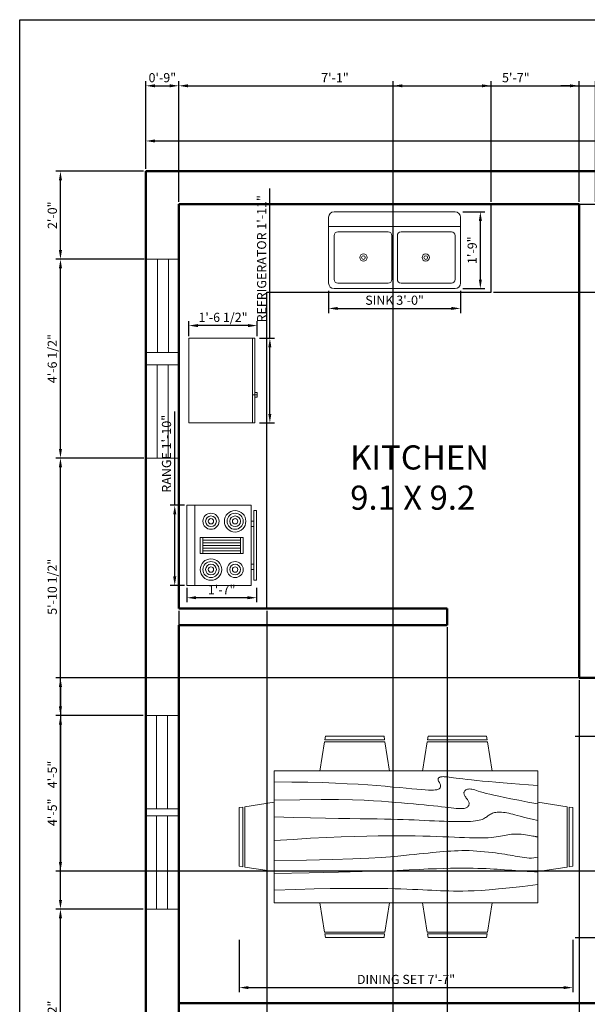
# Model space of a CAD drawing. Units: inches. Extents: x 231 to 633, y -1 to 510.
# Tile 2 of 3: x 231 to 386, y 242 to 510. Entities that reach past the tile are written whole.
import ezdxf

# ---------------------------------------------------------------- set-up
doc = ezdxf.new("R2010")
doc.units = ezdxf.units.IN
for name, color, linetype, lineweight in [('A-ANNO-DIMS', 2, 'Continuous', 18), ('A-ANNO-TTLB', 7, 'Continuous', 25), ('A-AREA-IDEN', 7, 'Continuous', 25), ('A-EQPM', 9, 'Continuous', 18), ('A-FLOR-CASE', 8, 'Continuous', 25), ('A-FLOR-FIXT', 9, 'Continuous', 18), ('A-FURN', 8, 'Continuous', 18), ('A-GLAZ', 4, 'Continuous', 18), ('A-WALL', 7, 'Continuous', 50)]:
    doc.layers.add(name, color=color, linetype=linetype, lineweight=lineweight)
doc.styles.get("Standard").update_dxf_attribs({"font": 'arial.ttf'})
doc.dimstyles.new('ISO-25', dxfattribs={"dimtxt": 2.5, "dimasz": 2.5, "dimexe": 1.25, "dimexo": 0.625, "dimtad": 1, "dimtxsty": 'Standard', "dimcen": 2.5, "dimadec": 0, "dimazin": 0, "dimtfac": 1, "dimtmove": 0, "dimatfit": 3, "dimfxl": 1, "dimarcsym": 0})

# ---------------------------------------------------------------- blocks, each defined once
blk = doc.blocks.new('Range-Oven - 30 in top')
for p, q in [((0, -3), (30, -3)), ((12, -6), (18, -6)), ((13, -20), (13, -6)), ((14, -6), (14, -20)), ((15, -20), (15, -6)), ((16, -6), (16, -20)), ((17, -20), (17, -6)), ((18, -20), (12, -20)), ((6, -24), (6, -25)), ((8, -25), (8, -24)), ((22, -25), (22, -24)), ((24, -24), (24, -25))]:
    blk.add_line(p, q)
for points in [[(0, -24), (0, 0), (30, 0), (30, -24)], [(12, -21), (12, -5), (18, -5), (18, -21)], [(2, -26), (2, -25), (28, -25), (28, -26)]]:
    blk.add_lwpolyline(points, close=True)
for centre, radius in [((6, -9), 4), ((6, -9), 3), ((6, -9), 2), ((24, -9), 3), ((24, -9), 2), ((6, -9), 1), ((24, -9), 1), ((24, -18), 4), ((6, -18), 3), ((6, -18), 2), ((6, -18), 1), ((24, -18), 3), ((24, -18), 2), ((24, -18), 1)]:
    blk.add_circle(centre, radius)
blk = doc.blocks.new('Refrigerator-2 door - 36 in top')
for p, q in [((0, -26.999999), (36, -26.999999)), ((11, -27.999999), (11, -28.999999)), ((11, -28.999999), (13, -28.999999)), ((12, -26.999999), (12, -28.999999)), ((13, -28.999999), (13, -27.999999))]:
    blk.add_line(p, q)
blk.add_lwpolyline([(0, -27.999999), (0, 0), (36, 0), (36, -27.999999)], close=True)
blk = doc.blocks.new('Sink-double - 36 in top')
for p, q in [((-18, -4), (18, -4)), ((-0.75, -18.5), (-0.75, -6.5)), ((0.75, -6.5), (0.75, -18.5))]:
    blk.add_line(p, q)
for points in [[(-16.5, 0), (16.5, 0)], [(-18, -19.5), (-18, -1.5)], [(18, -1.5), (18, -19.5)], [(-16.5, -18.5), (-16.5, -6.5)], [(-15.5, -5.5), (-1.75, -5.5)], [(1.75, -5.5), (15.5, -5.5)], [(16.5, -6.5), (16.5, -18.5)], [(16.5, -21), (-16.5, -21)], [(-1.75, -19.5), (-15.5, -19.5)], [(15.5, -19.5), (1.75, -19.5)]]:
    blk.add_lwpolyline(points)
for centre, radius in [((-8.5, -12.5), 1), ((-8.5, -12.5), 0.5), ((8.5, -12.5), 1), ((8.5, -12.5), 0.5)]:
    blk.add_circle(centre, radius)
for centre, radius, start, end in [((-16.5, -1.5), 1.5, 90, 180), ((16.5, -1.5), 1.5, 0, 90), ((-15.5, -6.5), 1, 90, 180), ((-1.75, -6.5), 1, 0, 90), ((1.75, -6.5), 1, 90, 180), ((15.5, -6.5), 1, 0, 90), ((-15.5, -18.5), 1, 180, 270), ((-1.75, -18.5), 1, 270, 0), ((1.75, -18.5), 1, 180, 270), ((15.5, -18.5), 1, 270, 0), ((-16.5, -19.5), 1.5, 180, 270), ((16.5, -19.5), 1.5, 270, 0)]:
    blk.add_arc(centre, radius, start, end)
blk = doc.blocks.new('Dining Set - 36 x 72 in.')
for p, q in [((-22, 27.5), (-22.1562, 26.50042)), ((-22, 27.5), (-6, 27.5)), ((-5.8437, 26.49966), (-6, 27.5)), ((6, 27.5), (5.8438, 26.50042)), ((6, 27.5), (22, 27.5)), ((22.1563, 26.49966), (22, 27.5)), ((-22.2343, 26.00059), (-23.4847, 17.99762)), ((-22.2304, 26), (-5.7608, 26)), ((-5.8416, 26.5), (-22.1534, 26.5)), ((-4.5152, 17.99762), (-5.7655, 25.99926)), ((5.7657, 26.00059), (4.5153, 17.99762)), ((5.7696, 26), (22.2392, 26)), ((22.1584, 26.5), (5.8466, 26.5)), ((23.4848, 17.99762), (22.2345, 25.99926)), ((36, 18), (-36, 18)), ((-36, 18), (-36, -18)), ((36, -18), (36, 18)), ((-45.5, 8), (-44.5004, 8.15617)), ((-44.5, -8.15843), (-44.5, 8.15338)), ((-44.0006, 8.23428), (-35.9976, 9.48474)), ((-44, 8.23041), (-44, -8.23915)), ((44.0006, 8.23428), (35.9976, 9.48474)), ((44, 8.23041), (44, -8.23915)), ((44.5, -8.15843), (44.5, 8.15338)), ((45.5, 8), (44.5005, 8.15617)), ((-45.5, 8), (-45.5, -8)), ((45.5, 8), (45.5, -8)), ((-44.4997, -8.15631), (-45.5, -8)), ((44.4997, -8.15631), (45.5, -8)), ((-35.9976, -9.48476), (-43.9993, -8.2345)), ((35.9976, -9.48476), (43.9993, -8.2345)), ((-36, -18), (36, -18)), ((-22.2343, -26.0006), (-23.4847, -17.99762)), ((-4.5152, -17.99762), (-5.7655, -25.99928)), ((5.7657, -26.0006), (4.5153, -17.99762)), ((23.4848, -17.99762), (22.2345, -25.99928)), ((-22.2304, -26), (-5.7608, -26)), ((-22, -27.5), (-22.1562, -26.50044)), ((-5.8416, -26.5), (-22.1534, -26.5)), ((-5.8437, -26.49967), (-6, -27.5)), ((5.7696, -26), (22.2392, -26)), ((6, -27.5), (5.8438, -26.50044)), ((22.1584, -26.5), (5.8466, -26.5)), ((22.1563, -26.49967), (22, -27.5)), ((-22, -27.5), (-6, -27.5)), ((6, -27.5), (22, -27.5))]:
    blk.add_line(p, q)
for points in [[(-36, 15), (-31.1772, 14.97754), (-26.8079, 14.91406), (-22.8538, 14.81543), (-19.276, 14.6875), (-16.0362, 14.53613), (-13.0957, 14.36718), (-10.4159, 14.18652), (-7.9583, 14), (-5.6904, 13.81315), (-3.6035, 13.63021), (-1.6954, 13.45508), (0.0365, 13.29166), (1.5945, 13.14388), (2.9811, 13.01562), (4.1988, 12.9108), (5.25, 12.83333), (6.1393, 12.78613), (6.8802, 12.76823), (7.4883, 12.77767), (7.9792, 12.8125), (8.3685, 12.87077), (8.6719, 12.95052), (8.9049, 13.0498), (9.0833, 13.16666), (9.2205, 13.29899), (9.3216, 13.44401), (9.3895, 13.59879), (9.4271, 13.76041), (9.4373, 13.92594), (9.4232, 14.09245), (9.3875, 14.257), (9.3333, 14.41666), (9.2638, 14.56917), (9.1836, 14.71484), (9.0975, 14.85465), (9.0104, 14.98958), (8.9272, 15.1206), (8.8529, 15.2487), (8.7922, 15.37483), (8.75, 15.5), (8.7305, 15.62467), (8.7344, 15.74739), (8.7617, 15.86621), (8.8125, 15.97916), (8.8867, 16.08431), (8.9844, 16.17968), (9.1055, 16.26334), (9.25, 16.33333), (9.4189, 16.38802), (9.6172, 16.42708), (9.8506, 16.45052), (10.125, 16.45833), (10.4463, 16.45052), (10.8203, 16.42708), (11.2529, 16.38802), (11.75, 16.33333), (12.3184, 16.26318), (12.9694, 16.17838), (13.7151, 16.07991), (14.5677, 15.96875), (15.5395, 15.84586), (16.6426, 15.71224), (17.8893, 15.56884), (19.2917, 15.41666), (20.859, 15.25667), (22.5879, 15.08984), (24.4721, 14.91715), (26.5052, 14.73958), (28.6809, 14.5581), (30.9929, 14.3737), (33.4347, 14.18733), (36, 14)], [(-36, 10), (-28.9766, 10.14274), (-23.1725, 10.20442), (-18.4241, 10.19775), (-14.5677, 10.13541), (-11.4399, 10.03011), (-8.877, 9.89453), (-6.7154, 9.74137), (-4.7917, 9.58333), (-2.9698, 9.43082), (-1.2246, 9.28515), (0.4415, 9.14534), (2.026, 9.01041), (3.5266, 8.87939), (4.9408, 8.7513), (6.266, 8.62516), (7.5, 8.5), (8.6411, 8.37549), (9.6914, 8.2539), (10.6538, 8.13818), (11.5312, 8.03125), (12.3267, 7.93603), (13.043, 7.85547), (13.6831, 7.79248), (14.25, 7.75), (14.7471, 7.7303), (15.1797, 7.73307), (15.5537, 7.75732), (15.875, 7.80208), (16.1494, 7.86637), (16.3828, 7.94922), (16.5811, 8.04964), (16.75, 8.16666), (16.8944, 8.29915), (17.0143, 8.44531), (17.1089, 8.60319), (17.1771, 8.77083), (17.218, 8.94629), (17.2305, 9.1276), (17.2137, 9.31282), (17.1667, 9.5), (17.0895, 9.6875), (16.987, 9.875), (16.8649, 10.0625), (16.7292, 10.25), (16.5856, 10.4375), (16.4401, 10.625), (16.2985, 10.8125), (16.1667, 11), (16.05, 11.18733), (15.9518, 11.3737), (15.8752, 11.5581), (15.8229, 11.73958), (15.798, 11.91715), (15.8034, 12.08984), (15.842, 12.25667), (15.9167, 12.41666), (16.0295, 12.56836), (16.1784, 12.70833), (16.3605, 12.83268), (16.5729, 12.9375), (16.8127, 13.01888), (17.0768, 13.07291), (17.3625, 13.0957), (17.6667, 13.08333), (17.9894, 13.03312), (18.3418, 12.94726), (18.7382, 12.82918), (19.1927, 12.68229), (19.7195, 12.51001), (20.3327, 12.31575), (21.0465, 12.10294), (21.875, 11.875), (22.8357, 11.63354), (23.959, 11.37304), (25.2786, 11.08618), (26.8282, 10.76562), (28.6414, 10.40405), (30.752, 9.99414), (33.1936, 9.52856), (36, 9)], [(-36, 5.5), (-30.7157, 5.3348), (-26.069, 5.20963), (-21.9946, 5.11767), (-18.4271, 5.05208), (-15.3009, 5.00602), (-12.5508, 4.97265), (-10.1112, 4.94515), (-7.9167, 4.91666), (-5.909, 4.88167), (-4.0586, 4.83984), (-2.3429, 4.79215), (-0.7396, 4.73958), (0.7739, 4.6831), (2.22, 4.6237), (3.6213, 4.56233), (5, 4.5), (6.373, 4.43782), (7.7344, 4.3776), (9.0723, 4.32129), (10.375, 4.27083), (11.6309, 4.22819), (12.8281, 4.19531), (13.9551, 4.17415), (15, 4.16666), (15.954, 4.17448), (16.819, 4.19791), (17.6001, 4.23698), (18.3021, 4.29166), (18.9299, 4.36198), (19.4883, 4.44791), (19.9823, 4.54948), (20.4167, 4.66666), (20.7969, 4.79899), (21.1302, 4.94401), (21.4245, 5.09879), (21.6875, 5.26041), (21.9271, 5.42594), (22.1511, 5.59245), (22.3672, 5.757), (22.5834, 5.91666), (22.8065, 6.06868), (23.0404, 6.21093), (23.2879, 6.34147), (23.5521, 6.45833), (23.8358, 6.55957), (24.142, 6.64323), (24.4735, 6.70735), (24.8334, 6.75), (25.2235, 6.76969), (25.642, 6.76692), (26.0858, 6.74267), (26.5521, 6.69791), (27.0379, 6.63362), (27.5404, 6.55078), (28.0565, 6.45036), (28.5834, 6.33333), (29.1242, 6.19987), (29.7071, 6.04687), (30.3661, 5.87044), (31.1354, 5.66666), (32.0493, 5.43164), (33.142, 5.16146), (34.4475, 4.85221), (36, 4.5)], [(-36, -1), (-30.7915, -0.6591), (-26.0195, -0.38216), (-21.6519, -0.16284), (-17.6563, 0.00521), (-14.0005, 0.12833), (-10.6523, 0.21289), (-7.5796, 0.26522), (-4.75, 0.29166), (-2.134, 0.29793), (0.2878, 0.28711), (2.5317, 0.26163), (4.6146, 0.22396), (6.5529, 0.17651), (8.3633, 0.12174), (10.0623, 0.06209), (11.6667, 0), (13.1899, -0.06201), (14.6341, -0.1211), (15.9982, -0.17432), (17.2813, -0.21875), (18.4823, -0.25147), (19.6003, -0.26953), (20.6343, -0.27002), (21.5834, -0.25), (22.4481, -0.20768), (23.2357, -0.14584), (23.9549, -0.06836), (24.6146, 0.02083), (25.2235, 0.11784), (25.7904, 0.21875), (26.3241, 0.31966), (26.8334, 0.41666), (27.3265, 0.50618), (27.8099, 0.58593), (28.2894, 0.65397), (28.7709, 0.70833), (29.2601, 0.74707), (29.763, 0.76823), (30.2855, 0.76985), (30.8334, 0.75), (31.4088, 0.70784), (31.9994, 0.64713), (32.589, 0.57275), (33.1615, 0.48958), (33.7008, 0.4025), (34.1908, 0.3164), (34.6153, 0.23616), (34.9584, 0.16666), (35.2099, 0.11165), (35.3848, 0.07031), (35.504, 0.04069), (35.5886, 0.02083), (35.6594, 0.00879), (35.7377, 0.0026), (35.8442, 0.00032), (36, 0)], [(-36, -6.5), (-27.1843, -6.31267), (-20.084, -6.1263), (-14.469, -5.9419), (-10.1094, -5.76042), (-6.7752, -5.58285), (-4.2363, -5.41016), (-2.2629, -5.24333), (-0.625, -5.08334), (0.8708, -4.93099), (2.2715, -4.78646), (3.5872, -4.64974), (4.8281, -4.52084), (6.0046, -4.39974), (7.127, -4.28646), (8.2053, -4.18099), (9.25, -4.08334), (10.2705, -3.99382), (11.2734, -3.91407), (12.2647, -3.84603), (13.25, -3.79167), (14.2354, -3.75293), (15.2266, -3.73177), (16.2295, -3.73015), (17.25, -3.75), (18.2912, -3.79248), (19.3451, -3.85547), (20.4009, -3.93604), (21.4479, -4.03125), (22.4754, -4.13819), (23.4727, -4.25391), (24.4289, -4.37549), (25.3334, -4.5), (26.1785, -4.62492), (26.9694, -4.74935), (27.7145, -4.87281), (28.4219, -4.99479), (29.1, -5.11483), (29.7572, -5.23242), (30.4016, -5.34709), (31.0417, -5.45834), (31.6837, -5.56437), (32.3262, -5.65821), (32.9658, -5.73153), (33.599, -5.77604), (34.2224, -5.78345), (34.8327, -5.74545), (35.4264, -5.65373), (36, -5.5)], [(-36, -10), (-26.4022, -9.81299), (-18.4675, -9.62891), (-11.9839, -9.45069), (-6.7396, -9.28125), (-2.5226, -9.12354), (0.8789, -8.98047), (3.6769, -8.85498), (6.0833, -8.75), (8.2767, -8.66765), (10.3021, -8.60677), (12.1712, -8.56543), (13.8958, -8.54167), (15.4876, -8.53353), (16.9583, -8.53907), (18.3197, -8.55632), (19.5834, -8.58334), (20.7616, -8.61841), (21.8685, -8.66081), (22.9188, -8.71004), (23.9271, -8.76563), (24.9081, -8.82707), (25.8763, -8.89388), (26.8465, -8.96558), (27.8334, -9.04167), (28.8474, -9.12118), (29.8828, -9.20117), (30.93, -9.27824), (31.9792, -9.34896), (33.0205, -9.40991), (34.0443, -9.45768), (35.0407, -9.48885), (36, -9.5)], [(-36, -14.5), (-30.0881, -14.33513), (-25.0332, -14.21224), (-20.7312, -14.12647), (-17.0781, -14.07292), (-13.97, -14.04671), (-11.3027, -14.04297), (-8.9724, -14.05681), (-6.875, -14.08334), (-4.9224, -14.11833), (-3.0905, -14.16016), (-1.3709, -14.20785), (0.2448, -14.26042), (1.7647, -14.3169), (3.1973, -14.3763), (4.5507, -14.43767), (5.8333, -14.5), (7.0554, -14.5621), (8.235, -14.62175), (9.3922, -14.67652), (10.5469, -14.72396), (11.7192, -14.76164), (12.929, -14.78711), (14.1965, -14.79794), (15.5417, -14.79167), (16.9933, -14.76424), (18.6152, -14.70508), (20.4804, -14.60197), (22.6615, -14.44271), (25.2312, -14.21509), (28.2624, -13.9069), (31.8277, -13.50594), (36, -13)]]:
    blk.add_lwpolyline(points)
blk = doc.blocks.new('*D10')
at = {"layer": 'A-ANNO-DIMS', "color": 0, "lineweight": -2, "transparency": 16777216}
for p, q in [((265.28, 469.66), (265.28, 478.56)), ((589.28, 469.66), (589.28, 478.56)), ((267.78, 477.31), (586.78, 477.31))]:
    blk.add_line(p, q, dxfattribs=at)
at = {"layer": 'A-ANNO-DIMS', "color": 0, "transparency": 16777216}
for points in [[(267.78, 477.73), (267.78, 476.89), (265.28, 477.31)], [(586.78, 477.73), (586.78, 476.89), (589.28, 477.31)]]:
    blk.add_solid(points, dxfattribs=at)
at = {"layer": 'Defpoints', "color": 0, "transparency": 16777216}
for p in [(589.28, 477.31), (265.28, 469.03), (589.28, 469.03)]:
    blk.add_point(p, dxfattribs=at)
at = {"layer": 'A-ANNO-DIMS', "color": 0, "transparency": 16777216, "insert": (427.28, 478.44), "char_height": 1, "attachment_point": 5}
blk.add_mtext("27'", dxfattribs=at)
blk = doc.blocks.new('WIN-25_43x9')
for p, q in [((0, 0), (0, 9)), ((0, 9), (25.43, 9)), ((25.43, 9), (25.43, 0)), ((25.43, 6), (0, 6)), ((0, 3), (25.43, 3)), ((25.43, 0), (0, 0))]:
    blk.add_line(p, q)
blk = doc.blocks.new('*D22')
at = {"layer": 'A-ANNO-DIMS', "color": 0, "lineweight": -2, "transparency": 16777216}
for p, q in [((273.16, 377.85), (273.16, 403.45)), ((275.83, 377.85), (271.91, 377.85)), ((273.16, 358.39), (273.16, 375.35)), ((275.83, 355.89), (271.91, 355.89))]:
    blk.add_line(p, q, dxfattribs=at)
at = {"layer": 'A-ANNO-DIMS', "color": 0, "transparency": 16777216}
for points in [[(272.74, 375.35), (273.58, 375.35), (273.16, 377.85)], [(272.74, 358.39), (273.58, 358.39), (273.16, 355.89)]]:
    blk.add_solid(points, dxfattribs=at)
at = {"layer": 'Defpoints', "color": 0, "transparency": 16777216}
for p in [(273.16, 377.85), (276.46, 377.85), (276.46, 355.89)]:
    blk.add_point(p, dxfattribs=at)
at = {"layer": 'A-ANNO-DIMS', "color": 0, "transparency": 16777216, "insert": (271.24, 391.9), "char_height": 2.5, "attachment_point": 5, "rotation": 90}
blk.add_mtext('RANGE 1\'-10"', dxfattribs=at)
blk = doc.blocks.new('*D23')
at = {"layer": 'A-ANNO-DIMS', "color": 0, "lineweight": -2, "transparency": 16777216}
for p, q in [((276.46, 355.26), (276.46, 351.34)), ((295.49, 355.26), (295.49, 351.34)), ((292.99, 352.59), (278.96, 352.59))]:
    blk.add_line(p, q, dxfattribs=at)
at = {"layer": 'A-ANNO-DIMS', "color": 0, "transparency": 16777216}
for points in [[(278.96, 353.01), (278.96, 352.18), (276.46, 352.59)], [(292.99, 353.01), (292.99, 352.18), (295.49, 352.59)]]:
    blk.add_solid(points, dxfattribs=at)
at = {"layer": 'Defpoints', "color": 0, "transparency": 16777216}
for p in [(276.46, 355.89), (295.49, 355.89), (276.46, 352.59)]:
    blk.add_point(p, dxfattribs=at)
at = {"layer": 'A-ANNO-DIMS', "color": 0, "transparency": 16777216, "insert": (285.97, 354.47), "char_height": 2.5, "attachment_point": 5}
blk.add_mtext('1\'-7"', dxfattribs=at)
blk = doc.blocks.new('*D24')
at = {"layer": 'A-ANNO-DIMS', "color": 0, "lineweight": -2, "transparency": 16777216}
for p, q in [((299.12, 423.43), (299.12, 464.35)), ((296.27, 423.43), (300.37, 423.43)), ((299.12, 402.8), (299.12, 420.93)), ((296.27, 400.3), (300.37, 400.3))]:
    blk.add_line(p, q, dxfattribs=at)
at = {"layer": 'A-ANNO-DIMS', "color": 0, "transparency": 16777216}
for points in [[(298.7, 420.93), (299.53, 420.93), (299.12, 423.43)], [(298.7, 402.8), (299.53, 402.8), (299.12, 400.3)]]:
    blk.add_solid(points, dxfattribs=at)
at = {"layer": 'Defpoints', "color": 0, "transparency": 16777216}
for p in [(295.65, 423.43), (299.12, 423.43), (295.65, 400.3)]:
    blk.add_point(p, dxfattribs=at)
at = {"layer": 'A-ANNO-DIMS', "color": 0, "transparency": 16777216, "insert": (297.2, 445.14), "char_height": 2.5, "attachment_point": 5, "rotation": 90}
blk.add_mtext('REFRIGERATOR 1\'-11"', dxfattribs=at)
blk = doc.blocks.new('*D25')
at = {"layer": 'A-ANNO-DIMS', "color": 0, "lineweight": -2, "transparency": 16777216}
for p, q in [((277.02, 424.05), (277.02, 428.15)), ((295.65, 424.05), (295.65, 428.15)), ((293.15, 426.9), (279.52, 426.9))]:
    blk.add_line(p, q, dxfattribs=at)
at = {"layer": 'A-ANNO-DIMS', "color": 0, "transparency": 16777216}
for points in [[(279.52, 427.31), (279.52, 426.48), (277.02, 426.9)], [(293.15, 427.31), (293.15, 426.48), (295.65, 426.9)]]:
    blk.add_solid(points, dxfattribs=at)
at = {"layer": 'Defpoints', "color": 0, "transparency": 16777216}
for p in [(277.02, 426.9), (277.02, 423.43), (295.65, 423.43)]:
    blk.add_point(p, dxfattribs=at)
at = {"layer": 'A-ANNO-DIMS', "color": 0, "transparency": 16777216, "insert": (286.33, 428.82), "char_height": 2.5, "attachment_point": 5}
blk.add_mtext('1\'-6 1/2"', dxfattribs=at)
blk = doc.blocks.new('*D26')
at = {"layer": 'A-ANNO-DIMS', "color": 0, "lineweight": -2, "transparency": 16777216}
for p, q in [((315.15, 436.36), (315.15, 430.33)), ((351.15, 436.36), (351.15, 430.33)), ((317.65, 431.58), (348.65, 431.58))]:
    blk.add_line(p, q, dxfattribs=at)
at = {"layer": 'A-ANNO-DIMS', "color": 0, "transparency": 16777216}
for points in [[(317.65, 432), (317.65, 431.17), (315.15, 431.58)], [(348.65, 432), (348.65, 431.17), (351.15, 431.58)]]:
    blk.add_solid(points, dxfattribs=at)
at = {"layer": 'Defpoints', "color": 0, "transparency": 16777216}
for p in [(315.15, 436.98), (351.15, 436.98), (351.15, 431.58)]:
    blk.add_point(p, dxfattribs=at)
at = {"layer": 'A-ANNO-DIMS', "color": 0, "transparency": 16777216, "insert": (333.15, 433.5), "char_height": 2.5, "attachment_point": 5}
blk.add_mtext('SINK 3\'-0"', dxfattribs=at)
blk = doc.blocks.new('*D27')
at = {"layer": 'A-ANNO-DIMS', "color": 0, "lineweight": -2, "transparency": 16777216}
for p, q in [((351.78, 457.98), (357.8, 457.98)), ((356.55, 439.48), (356.55, 455.48)), ((351.78, 436.98), (357.8, 436.98))]:
    blk.add_line(p, q, dxfattribs=at)
at = {"layer": 'A-ANNO-DIMS', "color": 0, "transparency": 16777216}
for points in [[(356.14, 455.48), (356.97, 455.48), (356.55, 457.98)], [(356.14, 439.48), (356.97, 439.48), (356.55, 436.98)]]:
    blk.add_solid(points, dxfattribs=at)
at = {"layer": 'Defpoints', "color": 0, "transparency": 16777216}
for p in [(351.15, 457.98), (356.55, 457.98), (351.15, 436.98)]:
    blk.add_point(p, dxfattribs=at)
at = {"layer": 'A-ANNO-DIMS', "color": 0, "transparency": 16777216, "insert": (354.65, 447.48), "char_height": 2.5, "attachment_point": 5, "rotation": 90}
blk.add_mtext('1\'-9"', dxfattribs=at)
blk = doc.blocks.new('*D28')
at = {"layer": 'A-ANNO-DIMS', "color": 0, "lineweight": -2, "transparency": 16777216}
for p, q in [((290.77, 259.16), (290.77, 244.88)), ((381.77, 259.16), (381.77, 244.88)), ((293.27, 246.13), (379.27, 246.13))]:
    blk.add_line(p, q, dxfattribs=at)
at = {"layer": 'A-ANNO-DIMS', "color": 0, "transparency": 16777216}
for points in [[(293.27, 246.55), (293.27, 245.72), (290.77, 246.13)], [(379.27, 246.55), (379.27, 245.72), (381.77, 246.13)]]:
    blk.add_solid(points, dxfattribs=at)
at = {"layer": 'Defpoints', "color": 0, "transparency": 16777216}
for p in [(290.77, 259.78), (381.77, 259.78), (381.77, 246.13)]:
    blk.add_point(p, dxfattribs=at)
at = {"layer": 'A-ANNO-DIMS', "color": 0, "transparency": 16777216, "insert": (336.27, 248.05), "char_height": 2.5, "attachment_point": 5}
blk.add_mtext('DINING SET 7\'-7"', dxfattribs=at)
blk = doc.blocks.new('*D29')
at = {"layer": 'A-ANNO-DIMS', "color": 0, "lineweight": -2, "transparency": 16777216}
for p, q in [((382.4, 314.78), (396.67, 314.78)), ((395.42, 262.28), (395.42, 312.28)), ((382.4, 259.78), (396.67, 259.78))]:
    blk.add_line(p, q, dxfattribs=at)
at = {"layer": 'A-ANNO-DIMS', "color": 0, "transparency": 16777216}
for points in [[(395.01, 312.28), (395.84, 312.28), (395.42, 314.78)], [(395.01, 262.28), (395.84, 262.28), (395.42, 259.78)]]:
    blk.add_solid(points, dxfattribs=at)
at = {"layer": 'Defpoints', "color": 0, "transparency": 16777216}
for p in [(381.77, 314.78), (395.42, 314.78), (381.77, 259.78)]:
    blk.add_point(p, dxfattribs=at)
at = {"layer": 'A-ANNO-DIMS', "color": 0, "transparency": 16777216, "insert": (393.55, 287.28), "char_height": 2.5, "attachment_point": 5, "rotation": 90}
blk.add_mtext('4\'-7"', dxfattribs=at)
blk = doc.blocks.new('*D34')
at = {"layer": 'A-ANNO-DIMS', "color": 0, "lineweight": -2, "transparency": 16777216}
for p, q in [((463.66, 330.73), (240.73, 330.73)), ((241.98, 328.23), (241.98, 280.43)), ((463.66, 277.93), (240.73, 277.93))]:
    blk.add_line(p, q, dxfattribs=at)
at = {"layer": 'A-ANNO-DIMS', "color": 0, "transparency": 16777216}
for points in [[(241.56, 328.23), (242.4, 328.23), (241.98, 330.73)], [(241.56, 280.43), (242.4, 280.43), (241.98, 277.93)]]:
    blk.add_solid(points, dxfattribs=at)
at = {"layer": 'Defpoints', "color": 0, "transparency": 16777216}
for p in [(464.28, 330.73), (241.98, 277.93), (464.28, 277.93)]:
    blk.add_point(p, dxfattribs=at)
at = {"layer": 'A-ANNO-DIMS', "color": 0, "transparency": 16777216, "insert": (240.08, 304.33), "char_height": 2.5, "attachment_point": 5, "rotation": 90}
blk.add_mtext('4\'-5"', dxfattribs=at)
blk = doc.blocks.new('*D37')
at = {"layer": 'A-ANNO-DIMS', "color": 0, "lineweight": -2, "transparency": 16777216}
for p, q in [((265.28, 469.66), (265.28, 493.62)), ((267.78, 492.37), (271.78, 492.37)), ((274.28, 460.66), (274.28, 493.62))]:
    blk.add_line(p, q, dxfattribs=at)
at = {"layer": 'A-ANNO-DIMS', "color": 0, "transparency": 16777216}
for points in [[(267.78, 492.78), (267.78, 491.95), (265.28, 492.37)], [(271.78, 492.78), (271.78, 491.95), (274.28, 492.37)]]:
    blk.add_solid(points, dxfattribs=at)
at = {"layer": 'Defpoints', "color": 0, "transparency": 16777216}
for p in [(274.28, 492.37), (265.28, 469.03), (274.28, 460.03)]:
    blk.add_point(p, dxfattribs=at)
at = {"layer": 'A-ANNO-DIMS', "color": 0, "transparency": 16777216, "insert": (269.78, 494.27), "char_height": 2.5, "attachment_point": 5}
blk.add_mtext('0\'-9"', dxfattribs=at)
blk = doc.blocks.new('*D38')
at = {"layer": 'A-ANNO-DIMS', "color": 0, "lineweight": -2, "transparency": 16777216}
for p, q in [((380.98, 492.37), (378.48, 492.37)), ((383.48, 460.66), (383.48, 493.62)), ((383.48, 492.37), (387.98, 492.37)), ((387.98, 460.66), (387.98, 493.62)), ((390.48, 492.37), (406.7, 492.37))]:
    blk.add_line(p, q, dxfattribs=at)
at = {"layer": 'A-ANNO-DIMS', "color": 0, "transparency": 16777216}
for points in [[(380.98, 492.78), (380.98, 491.95), (383.48, 492.37)], [(390.48, 492.78), (390.48, 491.95), (387.98, 492.37)]]:
    blk.add_solid(points, dxfattribs=at)
at = {"layer": 'Defpoints', "color": 0, "transparency": 16777216}
for p in [(387.98, 492.37), (383.48, 460.03), (387.98, 460.03)]:
    blk.add_point(p, dxfattribs=at)
at = {"layer": 'A-ANNO-DIMS', "color": 0, "transparency": 16777216, "insert": (399.84, 494.28), "char_height": 2.5, "attachment_point": 5}
blk.add_mtext('0\'-4 1/2"', dxfattribs=at)
blk = doc.blocks.new('*D39')
at = {"layer": 'A-ANNO-DIMS', "color": 0, "lineweight": -2, "transparency": 16777216}
for p, q in [((274.28, 460.66), (274.28, 493.62)), ((276.78, 492.37), (356.98, 492.37)), ((359.48, 460.66), (359.48, 493.62))]:
    blk.add_line(p, q, dxfattribs=at)
at = {"layer": 'A-ANNO-DIMS', "color": 0, "transparency": 16777216}
for points in [[(276.78, 492.78), (276.78, 491.95), (274.28, 492.37)], [(356.98, 492.78), (356.98, 491.95), (359.48, 492.37)]]:
    blk.add_solid(points, dxfattribs=at)
at = {"layer": 'Defpoints', "color": 0, "transparency": 16777216}
for p in [(359.48, 492.37), (274.28, 460.03), (359.48, 460.03)]:
    blk.add_point(p, dxfattribs=at)
at = {"layer": 'A-ANNO-DIMS', "color": 0, "transparency": 16777216, "insert": (316.88, 494.25), "char_height": 2.5, "attachment_point": 5}
blk.add_mtext('7\'-1"', dxfattribs=at)
blk = doc.blocks.new('*D40')
at = {"layer": 'A-ANNO-DIMS', "color": 0, "lineweight": -2, "transparency": 16777216}
for p, q in [((360.11, 460.03), (613.74, 460.03)), ((612.49, 457.53), (612.49, 438.53)), ((360.11, 436.03), (613.74, 436.03))]:
    blk.add_line(p, q, dxfattribs=at)
at = {"layer": 'A-ANNO-DIMS', "color": 0, "transparency": 16777216}
for points in [[(612.08, 457.53), (612.91, 457.53), (612.49, 460.03)], [(612.08, 438.53), (612.91, 438.53), (612.49, 436.03)]]:
    blk.add_solid(points, dxfattribs=at)
at = {"layer": 'Defpoints', "color": 0, "transparency": 16777216}
for p in [(359.48, 460.03), (359.48, 436.03), (612.49, 436.03)]:
    blk.add_point(p, dxfattribs=at)
at = {"layer": 'A-ANNO-DIMS', "color": 0, "transparency": 16777216, "insert": (610.59, 448.03), "char_height": 2.5, "attachment_point": 5, "rotation": 90}
blk.add_mtext('2\'-0"', dxfattribs=at)
blk = doc.blocks.new('*D41')
at = {"layer": 'A-ANNO-DIMS', "color": 0, "lineweight": -2, "transparency": 16777216}
for p, q in [((274.28, 349.01), (274.28, 4.58)), ((298.28, 349.01), (298.28, 4.58)), ((276.78, 5.83), (295.78, 5.83))]:
    blk.add_line(p, q, dxfattribs=at)
at = {"layer": 'A-ANNO-DIMS', "color": 0, "transparency": 16777216}
for points in [[(276.78, 6.25), (276.78, 5.42), (274.28, 5.83)], [(295.78, 6.25), (295.78, 5.42), (298.28, 5.83)]]:
    blk.add_solid(points, dxfattribs=at)
at = {"layer": 'Defpoints', "color": 0, "transparency": 16777216}
for p in [(274.28, 349.63), (298.28, 349.63), (298.28, 5.83)]:
    blk.add_point(p, dxfattribs=at)
at = {"layer": 'A-ANNO-DIMS', "color": 0, "transparency": 16777216, "insert": (286.28, 7.73), "char_height": 2.5, "attachment_point": 5}
blk.add_mtext('2\'-0"', dxfattribs=at)
blk = doc.blocks.new('*D42')
at = {"layer": 'A-ANNO-DIMS', "color": 0, "lineweight": -2, "transparency": 16777216}
for p, q in [((347.48, 344.51), (347.48, 4.58)), ((383.48, 330.11), (383.48, 4.58)), ((349.98, 5.83), (380.98, 5.83))]:
    blk.add_line(p, q, dxfattribs=at)
at = {"layer": 'A-ANNO-DIMS', "color": 0, "transparency": 16777216}
for points in [[(349.98, 6.25), (349.98, 5.42), (347.48, 5.83)], [(380.98, 6.25), (380.98, 5.42), (383.48, 5.83)]]:
    blk.add_solid(points, dxfattribs=at)
at = {"layer": 'Defpoints', "color": 0, "transparency": 16777216}
for p in [(347.48, 345.13), (383.48, 330.73), (383.48, 5.83)]:
    blk.add_point(p, dxfattribs=at)
at = {"layer": 'A-ANNO-DIMS', "color": 0, "transparency": 16777216, "insert": (365.48, 7.73), "char_height": 2.5, "attachment_point": 5}
blk.add_mtext('3\'-0"', dxfattribs=at)
blk = doc.blocks.new('*D45')
at = {"layer": 'A-ANNO-DIMS', "color": 0, "lineweight": -2, "transparency": 16777216}
for p, q in [((264.59, 267.58), (240.73, 267.58)), ((241.98, 206.66), (241.98, 265.08)), ((264.65, 204.16), (240.73, 204.16))]:
    blk.add_line(p, q, dxfattribs=at)
at = {"layer": 'A-ANNO-DIMS', "color": 0, "transparency": 16777216}
for points in [[(241.56, 265.08), (242.4, 265.08), (241.98, 267.58)], [(241.56, 206.66), (242.4, 206.66), (241.98, 204.16)]]:
    blk.add_solid(points, dxfattribs=at)
at = {"layer": 'Defpoints', "color": 0, "transparency": 16777216}
for p in [(241.98, 267.58), (265.22, 267.58), (265.27, 204.16)]:
    blk.add_point(p, dxfattribs=at)
at = {"layer": 'A-ANNO-DIMS', "color": 0, "transparency": 16777216, "insert": (240.06, 235.87), "char_height": 2.5, "attachment_point": 5, "rotation": 90}
blk.add_mtext('5\'-3 1/2"', dxfattribs=at)
blk = doc.blocks.new('*D46')
at = {"layer": 'A-ANNO-DIMS', "color": 0, "lineweight": -2, "transparency": 16777216}
for p, q in [((264.55, 320.42), (240.73, 320.42)), ((241.98, 270.08), (241.98, 317.92)), ((264.59, 267.58), (240.73, 267.58))]:
    blk.add_line(p, q, dxfattribs=at)
at = {"layer": 'A-ANNO-DIMS', "color": 0, "transparency": 16777216}
for points in [[(241.56, 317.92), (242.4, 317.92), (241.98, 320.42)], [(241.56, 270.08), (242.4, 270.08), (241.98, 267.58)]]:
    blk.add_solid(points, dxfattribs=at)
at = {"layer": 'Defpoints', "color": 0, "transparency": 16777216}
for p in [(241.98, 320.42), (265.18, 320.42), (265.22, 267.58)]:
    blk.add_point(p, dxfattribs=at)
at = {"layer": 'A-ANNO-DIMS', "color": 0, "transparency": 16777216, "insert": (240.08, 294), "char_height": 2.5, "attachment_point": 5, "rotation": 90}
blk.add_mtext('4\'-5"', dxfattribs=at)
blk = doc.blocks.new('*D47')
at = {"layer": 'A-ANNO-DIMS', "color": 0, "lineweight": -2, "transparency": 16777216}
for p, q in [((264.77, 390.74), (240.73, 390.74)), ((241.98, 322.92), (241.98, 388.24)), ((264.55, 320.42), (240.73, 320.42))]:
    blk.add_line(p, q, dxfattribs=at)
at = {"layer": 'A-ANNO-DIMS', "color": 0, "transparency": 16777216}
for points in [[(241.56, 388.24), (242.4, 388.24), (241.98, 390.74)], [(241.56, 322.92), (242.4, 322.92), (241.98, 320.42)]]:
    blk.add_solid(points, dxfattribs=at)
at = {"layer": 'Defpoints', "color": 0, "transparency": 16777216}
for p in [(241.98, 390.74), (265.4, 390.74), (265.18, 320.42)]:
    blk.add_point(p, dxfattribs=at)
at = {"layer": 'A-ANNO-DIMS', "color": 0, "transparency": 16777216, "insert": (240.06, 355.58), "char_height": 2.5, "attachment_point": 5, "rotation": 90}
blk.add_mtext('5\'-10 1/2"', dxfattribs=at)
blk = doc.blocks.new('*D48')
at = {"layer": 'A-ANNO-DIMS', "color": 0, "lineweight": -2, "transparency": 16777216}
for p, q in [((264.79, 445.01), (240.73, 445.01)), ((241.98, 393.24), (241.98, 442.51)), ((264.77, 390.74), (240.73, 390.74))]:
    blk.add_line(p, q, dxfattribs=at)
at = {"layer": 'A-ANNO-DIMS', "color": 0, "transparency": 16777216}
for points in [[(241.56, 442.51), (242.4, 442.51), (241.98, 445.01)], [(241.56, 393.24), (242.4, 393.24), (241.98, 390.74)]]:
    blk.add_solid(points, dxfattribs=at)
at = {"layer": 'Defpoints', "color": 0, "transparency": 16777216}
for p in [(241.98, 445.01), (265.42, 445.01), (265.4, 390.74)]:
    blk.add_point(p, dxfattribs=at)
at = {"layer": 'A-ANNO-DIMS', "color": 0, "transparency": 16777216, "insert": (240.06, 417.88), "char_height": 2.5, "attachment_point": 5, "rotation": 90}
blk.add_mtext('4\'-6 1/2"', dxfattribs=at)
blk = doc.blocks.new('*D49')
at = {"layer": 'A-ANNO-DIMS', "color": 0, "lineweight": -2, "transparency": 16777216}
for p, q in [((264.66, 469.03), (240.73, 469.03)), ((241.98, 447.51), (241.98, 466.53)), ((264.79, 445.01), (240.73, 445.01))]:
    blk.add_line(p, q, dxfattribs=at)
at = {"layer": 'A-ANNO-DIMS', "color": 0, "transparency": 16777216}
for points in [[(241.56, 466.53), (242.4, 466.53), (241.98, 469.03)], [(241.56, 447.51), (242.4, 447.51), (241.98, 445.01)]]:
    blk.add_solid(points, dxfattribs=at)
at = {"layer": 'Defpoints', "color": 0, "transparency": 16777216}
for p in [(241.98, 469.03), (265.28, 469.03), (265.42, 445.01)]:
    blk.add_point(p, dxfattribs=at)
at = {"layer": 'A-ANNO-DIMS', "color": 0, "transparency": 16777216, "insert": (240.08, 457.02), "char_height": 2.5, "attachment_point": 5, "rotation": 90}
blk.add_mtext('2\'-0"', dxfattribs=at)
blk = doc.blocks.new('*D65')
at = {"layer": 'A-ANNO-DIMS', "color": 0, "lineweight": -2, "transparency": 16777216}
for p, q in [((332.78, 116.86), (332.78, 493.62)), ((335.28, 492.37), (397.18, 492.37)), ((399.68, 116.86), (399.68, 493.62))]:
    blk.add_line(p, q, dxfattribs=at)
at = {"layer": 'A-ANNO-DIMS', "color": 0, "transparency": 16777216}
for points in [[(335.28, 492.78), (335.28, 491.95), (332.78, 492.37)], [(397.18, 492.78), (397.18, 491.95), (399.68, 492.37)]]:
    blk.add_solid(points, dxfattribs=at)
at = {"layer": 'Defpoints', "color": 0, "transparency": 16777216}
for p in [(399.68, 492.37), (332.78, 116.23), (399.68, 116.23)]:
    blk.add_point(p, dxfattribs=at)
at = {"layer": 'A-ANNO-DIMS', "color": 0, "transparency": 16777216, "insert": (366.23, 494.26), "char_height": 2.5, "attachment_point": 5}
blk.add_mtext('5\'-7"', dxfattribs=at)

msp = doc.modelspace()

# ---------------------------------------------------------------- linework, layer by layer
at = {"layer": 'A-ANNO-TTLB'}
msp.add_lwpolyline([(230.86, 510.42), (632.68, 510.42), (632.68, -0.86), (230.86, -0.86)], close=True, dxfattribs=at)
at = {"layer": 'A-FLOR-CASE'}
for p, q in [((359.48, 436.03), (359.48, 460.03)), ((274.28, 436.03), (274.42, 436.03)), ((298.28, 349.63), (298.28, 436.03)), ((298.28, 436.03), (359.48, 436.03))]:
    msp.add_line(p, q, dxfattribs=at)
at = {"layer": 'A-WALL'}
for p, q in [((265.28, 49.03), (265.28, 469.03)), ((265.28, 469.03), (589.28, 469.03)), ((274.28, 460.03), (383.48, 460.03)), ((274.28, 349.63), (274.28, 460.03)), ((383.48, 330.73), (383.48, 460.03)), ((274.28, 349.63), (347.48, 349.63)), ((347.48, 345.13), (347.48, 349.63)), ((274.28, 345.13), (347.48, 345.13)), ((274.28, 116.23), (274.28, 345.13)), ((383.48, 330.73), (387.98, 330.73)), ((274.28, 241.93), (420.38, 241.93))]:
    msp.add_line(p, q, dxfattribs=at)

# ---------------------------------------------------------------- block references
at = {"layer": 'A-EQPM', "rotation": 90}
for name, p, xscale, yscale, zscale in [('Refrigerator-2 door - 36 in top', (277.02, 400.3), 0.6424335555075315, 0.6424335555075315, 0.6424335555075315), ('Range-Oven - 30 in top', (276.46, 355.89), 0.7321923404332642, 0.7321923404332642, 0.7321923404332642)]:
    msp.add_blockref(name, p, dxfattribs=dict(at, xscale=xscale, yscale=yscale, zscale=zscale))
at = {"layer": 'A-FLOR-FIXT'}
msp.add_blockref('Sink-double - 36 in top', (333.15, 457.98), dxfattribs=at)
at = {"layer": 'A-FURN'}
msp.add_blockref('Dining Set - 36 x 72 in.', (336.27, 287.28), dxfattribs=at)
at = {"layer": 'A-GLAZ'}
for p, rotation in [((265.42, 445.01), 270.0000000000001), ((265.4, 416.17), 270.0000000000001), ((265.18, 320.42), 269.9999999999998), ((265.22, 293.01), 270.0000000000001)]:
    msp.add_blockref('WIN-25_43x9', p, dxfattribs=dict(at, rotation=rotation))

# ---------------------------------------------------------------- texts
at = {"layer": 'A-AREA-IDEN', "insert": (321.03, 394.19), "char_height": 6.588, "attachment_point": 1}
msp.add_mtext_dynamic_manual_height_columns('KITCHEN\\P9.1 X 9.2', width=138.4826, gutter_width=32.94, heights=[0], dxfattribs=at)

# ---------------------------------------------------------------- dimensions: what is measured, and where the dimension line sits
at = {"layer": 'A-ANNO-DIMS'}
for base, p1, p2, override, picture, middle in [((387.98, 492.37), (383.48, 460.03), (387.98, 460.03), {"dimdec": 1, "dimlfac": 1, "dimrnd": 0, "dimzin": 1, "dimdsep": 46, "dimlunit": 4, "dimfrac": 2}, '*D38', (399.84, 494.28)), ((274.28, 492.37), (265.28, 469.03), (274.28, 460.03), {"dimdec": 1, "dimlfac": 1, "dimrnd": 0, "dimzin": 1, "dimdsep": 46, "dimlunit": 4, "dimfrac": 2}, '*D37', (269.78, 494.27)), ((359.48, 492.37), (274.28, 460.03), (359.48, 460.03), {"dimdec": 1, "dimlfac": 1, "dimrnd": 0, "dimzin": 1, "dimdsep": 46, "dimlunit": 4, "dimfrac": 2}, '*D39', (316.88, 494.25)), ((399.68, 492.37), (332.78, 116.23), (399.68, 116.23), {"dimdec": 1, "dimlfac": 1, "dimrnd": 0, "dimzin": 1, "dimdsep": 46, "dimlunit": 4, "dimfrac": 2}, '*D65', (366.23, 494.26)), ((589.28, 477.31), (265.28, 469.03), (589.28, 469.03), {"dimtxt": 1, "dimdec": 0, "dimlunit": 3, "dimclrd": 0, "dimclre": 0, "dimclrt": 0, "dimtdec": 0}, '*D10', (427.28, 478.44)), ((298.28, 5.83), (274.28, 349.63), (298.28, 349.63), {"dimdec": 1, "dimlfac": 1, "dimrnd": 0, "dimzin": 1, "dimdsep": 46, "dimlunit": 4, "dimfrac": 2}, '*D41', (286.28, 7.73)), ((383.48, 5.83), (347.48, 345.13), (383.48, 330.73), {"dimdec": 1, "dimlfac": 1, "dimrnd": 0, "dimzin": 1, "dimdsep": 46, "dimlunit": 4, "dimfrac": 2}, '*D42', (365.48, 7.73))]:
    dim = msp.add_linear_dim(base=base, p1=p1, p2=p2, dimstyle='ISO-25', override=override, dxfattribs=at)
    dim.commit()
    dim.dimension.update_dxf_attribs({"geometry": picture, "text_midpoint": middle})
for base, p1, p2, angle, picture, middle in [((241.98, 469.03), (265.42, 445.01), (265.28, 469.03), 90, '*D49', (240.08, 457.02)), ((612.49, 436.03), (359.48, 460.03), (359.48, 436.03), 90, '*D40', (610.59, 448.03)), ((356.55, 457.98), (351.15, 436.98), (351.15, 457.98), 90, '*D27', (354.65, 447.48)), ((241.98, 445.01), (265.4, 390.74), (265.42, 445.01), 90, '*D48', (240.06, 417.88)), ((277.02, 426.9), (295.65, 423.43), (277.02, 423.43), 180, '*D25', (286.33, 428.82)), ((241.98, 390.74), (265.18, 320.42), (265.4, 390.74), 90, '*D47', (240.06, 355.58)), ((276.46, 352.59), (295.49, 355.89), (276.46, 355.89), 180, '*D23', (285.97, 354.47)), ((241.98, 277.93), (464.28, 330.73), (464.28, 277.93), 90, '*D34', (240.08, 304.33)), ((241.98, 320.42), (265.22, 267.58), (265.18, 320.42), 90, '*D46', (240.08, 294)), ((395.42, 314.78), (381.77, 259.78), (381.77, 314.78), 90, '*D29', (393.55, 287.28)), ((241.98, 267.58), (265.27, 204.16), (265.22, 267.58), 90, '*D45', (240.06, 235.87))]:
    dim = msp.add_linear_dim(base=base, p1=p1, p2=p2, angle=angle, dimstyle='ISO-25', override={"dimdec": 1, "dimlfac": 1, "dimrnd": 0, "dimzin": 1, "dimdsep": 46, "dimlunit": 4, "dimfrac": 2}, dxfattribs=at)
    dim.commit()
    dim.dimension.update_dxf_attribs({"geometry": picture, "text_midpoint": middle})
for base, p1, p2, text, picture, middle in [((299.12, 423.43), (295.65, 400.3), (295.65, 423.43), 'REFRIGERATOR <>', '*D24', (297.2, 445.14)), ((273.16, 377.85), (276.46, 355.89), (276.46, 377.85), 'RANGE <>', '*D22', (271.24, 391.9))]:
    dim = msp.add_linear_dim(base=base, p1=p1, p2=p2, angle=90, text=text, dimstyle='ISO-25', override={"dimdec": 1, "dimlfac": 1, "dimrnd": 0, "dimzin": 1, "dimdsep": 46, "dimlunit": 4, "dimfrac": 2}, dxfattribs=at)
    dim.commit()
    dim.dimension.update_dxf_attribs({"geometry": picture, "text_midpoint": middle})
for base, p1, p2, text, picture, middle in [((351.15, 431.58), (315.15, 436.98), (351.15, 436.98), 'SINK <>', '*D26', (333.15, 433.5)), ((381.77, 246.13), (290.77, 259.78), (381.77, 259.78), 'DINING SET <>', '*D28', (336.27, 248.05))]:
    dim = msp.add_linear_dim(base=base, p1=p1, p2=p2, text=text, dimstyle='ISO-25', override={"dimdec": 1, "dimlfac": 1, "dimrnd": 0, "dimzin": 1, "dimdsep": 46, "dimlunit": 4, "dimfrac": 2}, dxfattribs=at)
    dim.commit()
    dim.dimension.update_dxf_attribs({"geometry": picture, "text_midpoint": middle})

doc.saveas('drawing.dxf')
